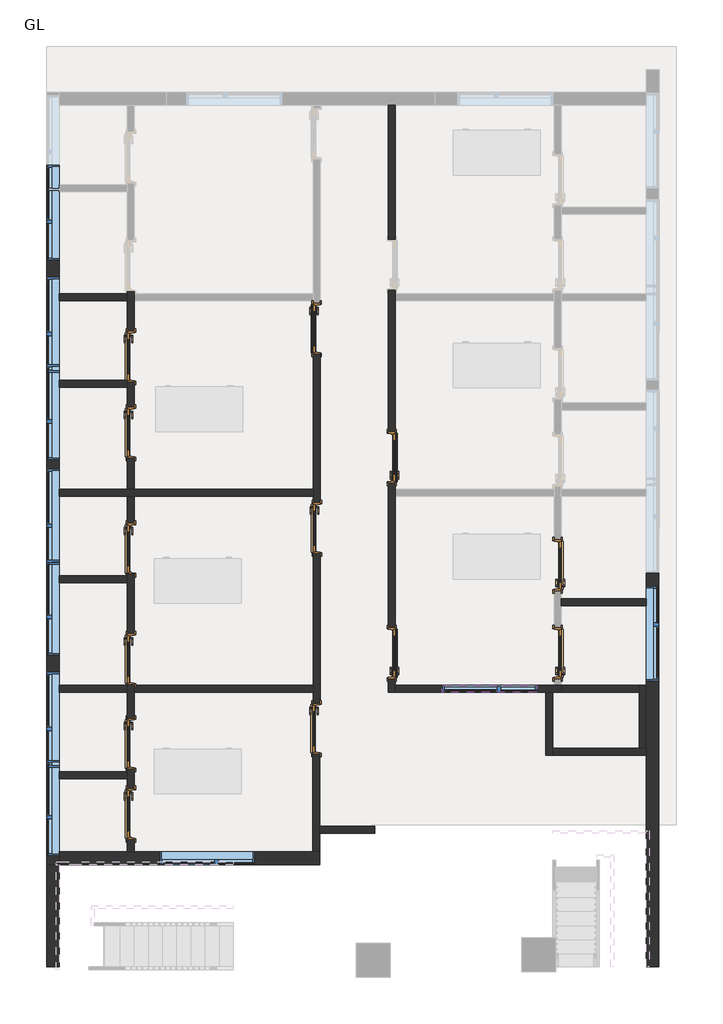
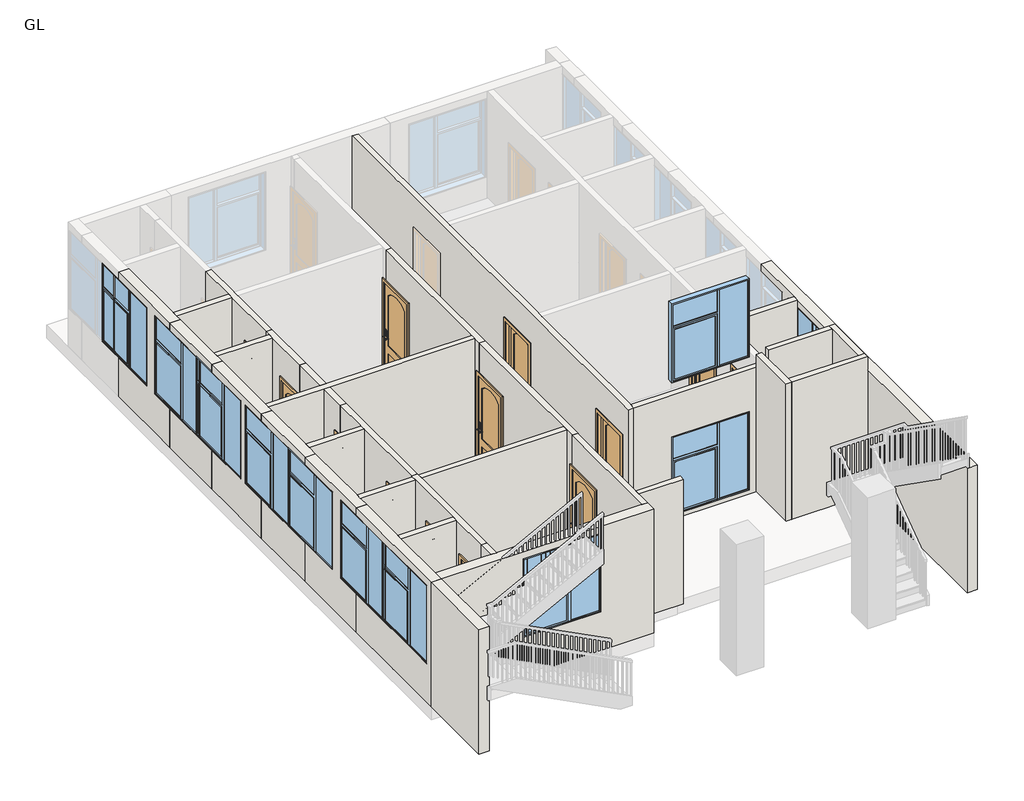
# One storey, part 1 of 4: 33 walls, 13 doors, 11 windows.
"""IFC4 building model written with IfcOpenShell, lengths in millimetres."""

from ifc_helpers import new_model, si_unit, frame, origin, origin_with_axes, place, context, project, spatial, polyline, outline, extrude, faceted_brep, transform, mapped, element, save
from components import door_346b4a94, m_window_casement_double_sidelight_1702_x_1829mm_c8b42c7f, m_window_casement_double_sidelight_1702_x_1829mm_92594323

model = new_model("IFC4")

# Units and contexts
model_context = context("Model", 3, world=origin())
ifc_project = project(units=[si_unit("LENGTHUNIT", "METRE", prefix="MILLI")], contexts=[model_context])

# Site, building, storey
site = spatial("IfcSite", under=ifc_project)
building = spatial("IfcBuilding", under=site)
storey = spatial("IfcBuildingStorey", under=building, Name="GL", Elevation=0.0)

# Doors
placement = place(None, origin())
door_shape = door_346b4a94(model_context)
element("IfcDoor", 1, ObjectType="2'10\"X7'", at=placement, inside=storey, context=model_context, shape_type="MappedRepresentation", body=[
    mapped(door_shape, transform((2698.7641134, -459.3600272, 0.0), x_axis=(0.0, -1.0, 0.0), y_axis=(1.0, 0.0, 0.0), z_axis=(0.0, 0.0, 1.0))),
])
element("IfcDoor", 2, ObjectType="2'10\"X7'", at=placement, inside=storey, context=model_context, shape_type="MappedRepresentation", body=[
    mapped(door_shape, transform((2698.7641134, -2034.1600272, 0.0), x_axis=(0.0, -1.0, 0.0), y_axis=(1.0, 0.0, 0.0), z_axis=(0.0, 0.0, 1.0))),
])
element("IfcDoor", 3, ObjectType="2'10\"X7'", at=placement, inside=storey, context=model_context, shape_type="MappedRepresentation", body=[
    mapped(door_shape, transform((-273.0358866, -2034.1600272, 0.0), x_axis=(0.0, -1.0, 0.0), y_axis=(1.0, 0.0, 0.0), z_axis=(0.0, 0.0, 1.0))),
])
element("IfcDoor", 4, ObjectType="2'10\"X7'", at=placement, inside=storey, context=model_context, shape_type="MappedRepresentation", body=[
    mapped(door_shape, transform((-273.0358866, 1471.0399728, 0.0), x_axis=(0.0, -1.0, 0.0), y_axis=(1.0, 0.0, 0.0), z_axis=(0.0, 0.0, 1.0))),
])
element("IfcDoor", 5, ObjectType="2'10\"X7'", at=placement, inside=storey, context=model_context, shape_type="MappedRepresentation", body=[
    mapped(door_shape, transform((-4952.9858866, -3659.7600272, 0.0), x_axis=(0.0, 1.0, 0.0), y_axis=(-1.0, 0.0, 0.0), z_axis=(0.0, 0.0, 1.0))),
])
element("IfcDoor", 6, ObjectType="2'10\"X7'", at=placement, inside=storey, context=model_context, shape_type="MappedRepresentation", body=[
    mapped(door_shape, transform((-4952.9858866, -2142.5151651, 0.0), x_axis=(0.0, 1.0, 0.0), y_axis=(-1.0, 0.0, 0.0), z_axis=(0.0, 0.0, 1.0))),
])
element("IfcDoor", 7, ObjectType="2'10\"X7'", at=placement, inside=storey, context=model_context, shape_type="MappedRepresentation", body=[
    mapped(door_shape, transform((-4952.9858866, -167.9704957, 0.0), x_axis=(0.0, 1.0, 0.0), y_axis=(-1.0, 0.0, 0.0), z_axis=(0.0, 0.0, 1.0))),
])
element("IfcDoor", 8, ObjectType="2'10\"X7'", at=placement, inside=storey, context=model_context, shape_type="MappedRepresentation", body=[
    mapped(door_shape, transform((-4952.9858866, 3273.6174518, 0.0), x_axis=(0.0, 1.0, 0.0), y_axis=(-1.0, 0.0, 0.0), z_axis=(0.0, 0.0, 1.0))),
])
element("IfcDoor", 9, ObjectType="2'10\"X7'", at=placement, inside=storey, context=model_context, shape_type="MappedRepresentation", body=[
    mapped(door_shape, transform((-1625.1621817, 3775.8008884, 0.0), x_axis=(0.0, 1.0, 0.0), y_axis=(-1.0, 0.0, 0.0), z_axis=(0.0, 0.0, 1.0))),
])
element("IfcDoor", 10, ObjectType="2'10\"X7'", at=placement, inside=storey, context=model_context, shape_type="MappedRepresentation", body=[
    mapped(door_shape, transform((-1629.1419858, -3390.4626067, 0.0), x_axis=(0.0, 1.0, 0.0), y_axis=(-1.0, 0.0, 0.0), z_axis=(0.0, 0.0, 1.0))),
])
element("IfcDoor", 11, ObjectType="2'10\"X7'", at=placement, inside=storey, context=model_context, shape_type="MappedRepresentation", body=[
    mapped(door_shape, transform((-1620.1577262, 202.9637706, 0.0), x_axis=(0.0, 1.0, 0.0), y_axis=(-1.0, 0.0, 0.0), z_axis=(0.0, 0.0, 1.0))),
])
element("IfcDoor", 12, ObjectType="2'10\"X7'", at=placement, inside=storey, context=model_context, shape_type="MappedRepresentation", body=[
    mapped(door_shape, transform((-4952.9858866, -4917.0600272, 0.0), x_axis=(0.0, 1.0, 0.0), y_axis=(-1.0, 0.0, 0.0), z_axis=(0.0, 0.0, 1.0))),
])
element("IfcDoor", 13, ObjectType="2'10\"X7'", at=placement, inside=storey, context=model_context, shape_type="MappedRepresentation", body=[
    mapped(door_shape, transform((-4952.9858866, 1913.3521609, 0.0), x_axis=(0.0, 1.0, 0.0), y_axis=(-1.0, 0.0, 0.0), z_axis=(0.0, 0.0, 1.0))),
])

# Walls
element("IfcWall", 14, ObjectType="Generic - 4.5\"", at=placement, inside=storey, context=model_context, shape_type="SweptSolid", body=[
    extrude(outline(polyline([(-5013.3108866, 4277.7399728), (-6232.5508078, 4277.7399728), (-6232.5508078, 4404.7399728), (-5013.3108866, 4404.7399728), (-5013.3108866, 4277.7399728)])), origin_with_axes(), (0.0, 0.0, 1.0), 2895.6),
])
element("IfcWall", 15, ObjectType="Generic - 4.5\"", at=placement, inside=storey, context=model_context, shape_type="Brep", body=[
    faceted_brep([(-5013.3108866, 2968.8174518, 2158.6), (-5013.3108866, 2968.8174518, 2895.6), (-5013.3108866, 4277.7399728, 2895.6), (-5013.3108866, 4404.7399728, 2895.6), (-5013.3108866, 5281.320652, 2895.6), (-5013.3108866, 5281.320652, 2158.6), (-5013.3108866, 4443.520652, 2158.6), (-5013.3108866, 4443.520652, 0.0), (-5013.3108866, 4404.7399728, 0.0), (-5013.3108866, 4277.7399728, 0.0), (-5013.3108866, 3730.4174518, 0.0), (-5013.3108866, 3730.4174518, 2158.6), (-4886.3108866, 2968.8174518, 2895.6), (-4886.3108866, 2968.8174518, 2158.6), (-4886.3108866, 3730.4174518, 2158.6), (-4886.3108866, 3730.4174518, 0.0), (-4886.3108866, 4277.7399728, 0.0), (-4886.3108866, 4404.7399728, 0.0), (-4886.3108866, 4443.520652, 0.0), (-4886.3108866, 4443.520652, 2158.6), (-4886.3108866, 5281.320652, 2158.6), (-4886.3108866, 5281.320652, 2895.6), (-4886.3108866, 4404.7399728, 2895.6), (-4886.3108866, 4277.7399728, 2895.6)], [[[0, 1, 2, 3, 4, 5, 6, 7, 8, 9, 10, 11]], [[12, 13, 14, 15, 16, 17, 18, 19, 20, 21, 22, 23]], [[15, 10, 9, 8, 7, 18, 17, 16]], [[1, 0, 13, 12]], [[4, 21, 20, 5]], [[14, 11, 10, 15]], [[11, 14, 13, 0]], [[19, 6, 5, 20]], [[6, 19, 18, 7]], [[4, 3, 2, 1, 12, 23, 22, 21]]]),
])
element("IfcWall", 16, ObjectType="Generic - 4.5\"", at=placement, inside=storey, context=model_context, shape_type="Brep", body=[
    faceted_brep([(-6232.5508078, 2728.3399728, 0.0), (-5013.3108866, 2728.3399728, 0.0), (-5013.3108866, 2728.3399728, 2895.6), (-6232.5508078, 2728.3399728, 2895.6), (-6232.5508078, 2855.3399728, 0.0), (-6232.5508078, 2855.3399728, 2895.6), (-5013.3108866, 2855.3399728, 2895.6), (-5013.3108866, 2855.3399728, 0.0), (-5013.3108866, 2816.8174518, 0.0)], [[[0, 1, 2, 3]], [[4, 5, 6, 7]], [[1, 0, 4, 7, 8]], [[0, 3, 5, 4]], [[2, 1, 8, 7, 6]], [[3, 2, 6, 5]]]),
])
element("IfcWall", 17, ObjectType="Generic - 4.5\"", at=placement, inside=storey, context=model_context, shape_type="Brep", body=[
    faceted_brep([(-5013.3108866, 2968.8174518, 2895.6), (-5013.3108866, 2968.8174518, 2158.6), (-5013.3108866, 2816.8174518, 2158.6), (-5013.3108866, 2816.8174518, 0.0), (-5013.3108866, 2728.3399728, 0.0), (-5013.3108866, 2370.1521609, 0.0), (-5013.3108866, 2370.1521609, 2158.6), (-5013.3108866, 1684.7521609, 2158.6), (-5013.3108866, 1684.7521609, 2895.6), (-5013.3108866, 2728.3399728, 2895.6), (-5013.3108866, 2855.3399728, 2895.6), (-4886.3108866, 2968.8174518, 2158.6), (-4886.3108866, 2968.8174518, 2895.6), (-4886.3108866, 1684.7521609, 2895.6), (-4886.3108866, 1684.7521609, 2158.6), (-4886.3108866, 2370.1521609, 2158.6), (-4886.3108866, 2370.1521609, 0.0), (-4886.3108866, 2816.8174518, 0.0), (-4886.3108866, 2816.8174518, 2158.6)], [[[0, 1, 2, 3, 4, 5, 6, 7, 8, 9, 10]], [[11, 12, 13, 14, 15, 16, 17, 18]], [[3, 17, 16, 5, 4]], [[13, 8, 7, 14]], [[1, 0, 12, 11]], [[18, 2, 1, 11]], [[2, 18, 17, 3]], [[15, 6, 5, 16]], [[6, 15, 14, 7]], [[0, 10, 9, 8, 13, 12]]]),
])
element("IfcWall", 18, ObjectType="Generic - 4.5\"", at=placement, inside=storey, context=model_context, shape_type="Brep", body=[
    faceted_brep([(-6232.5508078, 772.5399728, 0.0), (-5013.3108866, 772.5399728, 0.0), (-4886.3108866, 772.5399728, 0.0), (-1685.9108866, 772.5399728, 0.0), (-1685.9108866, 772.5399728, 2895.6), (-4886.3108866, 772.5399728, 2895.6), (-5013.3108866, 772.5399728, 2895.6), (-6232.5508078, 772.5399728, 2895.6), (-6232.5508078, 899.5399728, 0.0), (-6232.5508078, 899.5399728, 2895.6), (-5013.3108866, 899.5399728, 2895.6), (-4886.3108866, 899.5399728, 2895.6), (-1685.9108866, 899.5399728, 2895.6), (-1685.9108866, 899.5399728, 0.0), (-4886.3108866, 899.5399728, 0.0), (-5013.3108866, 899.5399728, 0.0)], [[[0, 1, 2, 3, 4, 5, 6, 7]], [[8, 9, 10, 11, 12, 13, 14, 15]], [[3, 2, 1, 0, 8, 15, 14, 13]], [[4, 3, 13, 12]], [[0, 7, 9, 8]], [[7, 6, 5, 4, 12, 11, 10, 9]]]),
])
element("IfcWall", 19, ObjectType="Generic - 4.5\"", at=placement, inside=storey, context=model_context, shape_type="SweptSolid", body=[
    extrude(outline(polyline([(136.8295043, 2158.6), (136.8295043, 2895.6), (772.5399728, 2895.6), (772.5399728, 0.0), (288.8295043, 0.0), (288.8295043, 2158.6), (136.8295043, 2158.6)])), frame((-5013.3108866, 0.0, 0.0), z_axis=(1.0, 0.0, 0.0), x_axis=(0.0, 1.0, 0.0)), (0.0, 0.0, 1.0), 127.0),
    extrude(outline(polyline([(1684.7521609, 2895.6), (1684.7521609, 2158.6), (1456.5521609, 2158.6), (1456.5521609, 0.0), (899.5399728, 0.0), (899.5399728, 2895.6), (1684.7521609, 2895.6)])), frame((-5013.3108866, 0.0, 0.0), z_axis=(1.0, 0.0, 0.0), x_axis=(0.0, 1.0, 0.0)), (0.0, 0.0, 1.0), 127.0),
])
element("IfcWall", 20, ObjectType="Generic - 4.5\"", at=placement, inside=storey, context=model_context, shape_type="SweptSolid", body=[
    extrude(outline(polyline([(-5013.3108866, -776.8600272), (-6232.5508078, -776.8600272), (-6232.5508078, -649.8600272), (-5013.3108866, -649.8600272), (-5013.3108866, -776.8600272)])), origin_with_axes(), (0.0, 0.0, 1.0), 2895.6),
])
element("IfcWall", 21, ObjectType="Generic - 4.5\"", at=placement, inside=storey, context=model_context, shape_type="Brep", body=[
    faceted_brep([(-5013.3108866, -2574.3151651, 2158.6), (-5013.3108866, -2574.3151651, 2895.6), (-5013.3108866, -776.8600272, 2895.6), (-5013.3108866, -649.8600272, 2895.6), (-5013.3108866, 136.8295043, 2895.6), (-5013.3108866, 136.8295043, 2158.6), (-5013.3108866, -624.7704957, 2158.6), (-5013.3108866, -624.7704957, 0.0), (-5013.3108866, -649.8600272, 0.0), (-5013.3108866, -776.8600272, 0.0), (-5013.3108866, -1685.7151651, 0.0), (-5013.3108866, -1685.7151651, 2158.6), (-4886.3108866, -2574.3151651, 2895.6), (-4886.3108866, -2574.3151651, 2158.6), (-4886.3108866, -1685.7151651, 2158.6), (-4886.3108866, -1685.7151651, 0.0), (-4886.3108866, -624.7704957, 0.0), (-4886.3108866, -624.7704957, 2158.6), (-4886.3108866, 136.8295043, 2158.6), (-4886.3108866, 136.8295043, 2895.6)], [[[0, 1, 2, 3, 4, 5, 6, 7, 8, 9, 10, 11]], [[12, 13, 14, 15, 16, 17, 18, 19]], [[15, 10, 9, 8, 7, 16]], [[1, 0, 13, 12]], [[4, 19, 18, 5]], [[14, 11, 10, 15]], [[11, 14, 13, 0]], [[17, 6, 5, 18]], [[6, 17, 16, 7]], [[4, 3, 2, 1, 12, 19]]]),
])
element("IfcWall", 22, ObjectType="Generic - 4.5\"", at=placement, inside=storey, context=model_context, shape_type="SweptSolid", body=[
    extrude(outline(polyline([(-5013.3108866, -2732.6600272), (-6232.5508078, -2732.6600272), (-6232.5508078, -2605.6600272), (-5013.3108866, -2605.6600272), (-5013.3108866, -2732.6600272)])), origin_with_axes(), (0.0, 0.0, 1.0), 2895.6),
])
element("IfcWall", 23, ObjectType="Generic - 4.5\"", at=placement, inside=storey, context=model_context, shape_type="Brep", body=[
    faceted_brep([(-5013.3108866, -3202.9600272, 0.0), (-5013.3108866, -3202.9600272, 2158.6), (-5013.3108866, -4116.5600272, 2158.6), (-5013.3108866, -4116.5600272, 0.0), (-5013.3108866, -4155.0600272, 0.0), (-5013.3108866, -4282.0600272, 0.0), (-5013.3108866, -4460.2600272, 0.0), (-5013.3108866, -4460.2600272, 2158.6), (-5013.3108866, -5221.8600272, 2158.6), (-5013.3108866, -5221.8600272, 2895.6), (-5013.3108866, -4282.0600272, 2895.6), (-5013.3108866, -4155.0600272, 2895.6), (-5013.3108866, -2732.6600272, 2895.6), (-5013.3108866, -2605.6600272, 2895.6), (-5013.3108866, -2574.3151651, 2895.6), (-5013.3108866, -2574.3151651, 2158.6), (-5013.3108866, -2599.3151651, 2158.6), (-5013.3108866, -2599.3151651, 0.0), (-5013.3108866, -2605.6600272, 0.0), (-5013.3108866, -2732.6600272, 0.0), (-4886.3108866, -3202.9600272, 2158.6), (-4886.3108866, -3202.9600272, 0.0), (-4886.3108866, -2732.6600272, 0.0), (-4886.3108866, -2605.6600272, 0.0), (-4886.3108866, -2599.3151651, 0.0), (-4886.3108866, -2599.3151651, 2158.6), (-4886.3108866, -2574.3151651, 2158.6), (-4886.3108866, -2574.3151651, 2895.6), (-4886.3108866, -2605.6600272, 2895.6), (-4886.3108866, -2732.6600272, 2895.6), (-4886.3108866, -5221.8600272, 2895.6), (-4886.3108866, -5221.8600272, 2158.6), (-4886.3108866, -4460.2600272, 2158.6), (-4886.3108866, -4460.2600272, 0.0), (-4886.3108866, -4116.5600272, 0.0), (-4886.3108866, -4116.5600272, 2158.6)], [[[0, 1, 2, 3, 4, 5, 6, 7, 8, 9, 10, 11, 12, 13, 14, 15, 16, 17, 18, 19]], [[20, 21, 22, 23, 24, 25, 26, 27, 28, 29, 30, 31, 32, 33, 34, 35]], [[21, 0, 19, 18, 17, 24, 23, 22]], [[3, 34, 33, 6, 5, 4]], [[30, 9, 8, 31]], [[15, 14, 27, 26]], [[20, 1, 0, 21]], [[1, 20, 35, 2]], [[2, 35, 34, 3]], [[25, 16, 15, 26]], [[16, 25, 24, 17]], [[32, 7, 6, 33]], [[7, 32, 31, 8]], [[14, 13, 12, 11, 10, 9, 30, 29, 28, 27]]]),
])
element("IfcWall", 24, ObjectType="Generic - 4.5\"", at=placement, inside=storey, context=model_context, shape_type="SweptSolid", body=[
    extrude(outline(polyline([(-5013.3108866, -4282.0600272), (-6232.5324766, -4282.0600272), (-6232.5342541, -4155.0600272), (-5013.3108866, -4155.0600272), (-5013.3108866, -4282.0600272)])), origin_with_axes(), (0.0, 0.0, 1.0), 2895.6),
])
element("IfcWall", 25, ObjectType="Generic - 4.5\"", at=placement, inside=storey, context=model_context, shape_type="SweptSolid", body=[
    extrude(outline(polyline([(-1685.9108866, -2732.6600272), (-4886.3108866, -2732.6600272), (-4886.3108866, -2605.6600272), (-1685.9108866, -2605.6600272), (-1685.9108866, -2732.6600272)])), origin_with_axes(), (0.0, 0.0, 1.0), 2895.6),
])
element("IfcWall", 26, ObjectType="Generic - 4.5\"", at=placement, inside=storey, context=model_context, shape_type="Brep", body=[
    faceted_brep([(-1685.4871817, 4182.2008884, 2895.6), (-1685.4871817, 4182.2008884, 2158.6), (-1685.4871817, 3319.0008884, 2158.6), (-1685.4871817, 3319.0008884, 0.0), (-1685.4871817, 659.7637706, 0.0), (-1685.4871817, 659.7637706, 2158.6), (-1685.4871817, 609.3637706, 2158.6), (-1685.4871817, 609.3637706, 2895.6), (-1558.4871817, 4182.2008884, 2158.6), (-1558.4871817, 4182.2008884, 2895.6), (-1558.4871817, 609.3637706, 2895.6), (-1558.4871817, 609.3637706, 2158.6), (-1558.4871817, 659.7637706, 2158.6), (-1558.4871817, 659.7637706, 0.0), (-1558.4871817, 3319.0008884, 0.0), (-1558.4871817, 3319.0008884, 2158.6), (-1680.4827262, 609.3637706, 2895.6), (-1680.4827262, 609.3637706, 2158.6), (-1558.9108866, 4182.2008884, 2895.6), (-1558.9108866, 4182.2008884, 2158.6)], [[[0, 1, 2, 3, 4, 5, 6, 7]], [[8, 9, 10, 11, 12, 13, 14, 15]], [[3, 14, 13, 4]], [[10, 16, 7, 6, 17, 11]], [[1, 0, 18, 9, 8, 19]], [[15, 2, 1, 19, 8]], [[2, 15, 14, 3]], [[12, 5, 4, 13]], [[5, 12, 11, 17, 6]], [[0, 7, 16, 10, 9, 18]]]),
])
element("IfcWall", 27, ObjectType="Generic - 4.5\"", at=placement, inside=storey, context=model_context, shape_type="Brep", body=[
    faceted_brep([(-1680.4827262, -2933.2626067, 0.0), (-1680.4827262, -2933.2626067, 2895.6), (-1680.4827262, 609.3637706, 2895.6), (-1680.4827262, 609.3637706, 2158.6), (-1680.4827262, -253.8362294, 2158.6), (-1680.4827262, -253.8362294, 0.0), (-1553.4827262, -2933.2626067, 2895.6), (-1553.4827262, -2933.2626067, 0.0), (-1553.4827262, -253.8362294, 0.0), (-1553.4827262, -253.8362294, 2158.6), (-1553.4827262, 609.3637706, 2158.6), (-1553.4827262, 609.3637706, 2895.6), (-1562.4669858, -2933.2626067, 0.0), (-1562.4669858, -2933.2626067, 2895.6), (-1558.4871817, 609.3637706, 2895.6), (-1558.4871817, 609.3637706, 2158.6)], [[[0, 1, 2, 3, 4, 5]], [[6, 7, 8, 9, 10, 11]], [[7, 12, 0, 5, 8]], [[1, 0, 12, 7, 6, 13]], [[2, 14, 11, 10, 15, 3]], [[9, 4, 3, 15, 10]], [[4, 9, 8, 5]], [[2, 1, 13, 6, 11, 14]]]),
])
element("IfcWall", 28, ObjectType="Generic - 4.5\"", at=placement, inside=storey, context=model_context, shape_type="Brep", body=[
    faceted_brep([(-1689.4669858, -2933.2626067, 2895.6), (-1689.4669858, -2933.2626067, 0.0), (-1689.4669858, -2933.6626067, 0.0), (-1689.4669858, -2933.6626067, 2158.6), (-1689.4669858, -3847.2626067, 2158.6), (-1689.4669858, -3847.2626067, 0.0), (-1689.4669858, -5596.1082131, 0.0), (-1689.4669858, -5596.1082131, 2895.6), (-1562.4669858, -2933.2626067, 0.0), (-1562.4669858, -2933.2626067, 2895.6), (-1562.4669858, -5136.3822004, 2895.6), (-1562.4669858, -5263.3822004, 2895.6), (-1562.4669858, -5596.1082131, 2895.6), (-1562.4669858, -5596.1082131, 0.0), (-1562.4669858, -5263.3822004, 0.0), (-1562.4669858, -5136.3822004, 0.0), (-1562.4669858, -3847.2626067, 0.0), (-1562.4669858, -3847.2626067, 2158.6), (-1562.4669858, -2933.6626067, 2158.6), (-1562.4669858, -2933.6626067, 0.0), (-1680.4827262, -2933.2626067, 0.0), (-1680.4827262, -2933.2626067, 2895.6)], [[[0, 1, 2, 3, 4, 5, 6, 7]], [[8, 9, 10, 11, 12, 13, 14, 15, 16, 17, 18, 19]], [[1, 20, 8, 19, 2]], [[13, 6, 5, 16, 15, 14]], [[1, 0, 21, 9, 8, 20]], [[18, 3, 2, 19]], [[3, 18, 17, 4]], [[4, 17, 16, 5]], [[7, 6, 13, 12]], [[0, 7, 12, 11, 10, 9, 21]]]),
])
element("IfcWall", 29, ObjectType="Generic - 4.5\"", at=placement, inside=storey, context=model_context, shape_type="Brep", body=[
    faceted_brep([(-339.7108866, 7782.9399728, 2895.6), (-339.7108866, 7782.9399728, 0.0), (-339.7108866, 5382.2399728, 0.0), (-339.7108866, 5382.2399728, 2158.6), (-339.7108866, 4468.6399728, 2158.6), (-339.7108866, 4468.6399728, 0.0), (-339.7108866, 1927.8399728, 0.0), (-339.7108866, 1927.8399728, 2158.6), (-339.7108866, 1014.2399728, 2158.6), (-339.7108866, 1014.2399728, 0.0), (-339.7108866, -1577.3600272, 0.0), (-339.7108866, -1577.3600272, 2158.6), (-339.7108866, -2490.9600272, 2158.6), (-339.7108866, -2490.9600272, 0.0), (-339.7108866, -2732.6600272, 0.0), (-339.7108866, -2732.6600272, 2895.6), (-212.7108866, 7782.9399728, 0.0), (-212.7108866, 7782.9399728, 2895.6), (-212.7108866, 4404.7399728, 2895.6), (-212.7108866, 4277.7399728, 2895.6), (-212.7108866, 899.5399728, 2895.6), (-212.7108866, 772.5399728, 2895.6), (-212.7108866, -2605.6600272, 2895.6), (-212.7108866, -2732.6600272, 2895.6), (-212.7108866, -2732.6600272, 0.0), (-212.7108866, -2605.6600272, 0.0), (-212.7108866, -2490.9600272, 0.0), (-212.7108866, -2490.9600272, 2158.6), (-212.7108866, -1577.3600272, 2158.6), (-212.7108866, -1577.3600272, 0.0), (-212.7108866, 772.5399728, 0.0), (-212.7108866, 899.5399728, 0.0), (-212.7108866, 1014.2399728, 0.0), (-212.7108866, 1014.2399728, 2158.6), (-212.7108866, 1927.8399728, 2158.6), (-212.7108866, 1927.8399728, 0.0), (-212.7108866, 4277.7399728, 0.0), (-212.7108866, 4404.7399728, 0.0), (-212.7108866, 4468.6399728, 0.0), (-212.7108866, 4468.6399728, 2158.6), (-212.7108866, 5382.2399728, 2158.6), (-212.7108866, 5382.2399728, 0.0)], [[[0, 1, 2, 3, 4, 5, 6, 7, 8, 9, 10, 11, 12, 13, 14, 15]], [[16, 17, 18, 19, 20, 21, 22, 23, 24, 25, 26, 27, 28, 29, 30, 31, 32, 33, 34, 35, 36, 37, 38, 39, 40, 41]], [[1, 16, 41, 2]], [[24, 14, 13, 26, 25]], [[29, 10, 9, 32, 31, 30]], [[35, 6, 5, 38, 37, 36]], [[1, 0, 17, 16]], [[15, 14, 24, 23]], [[12, 27, 26, 13]], [[27, 12, 11, 28]], [[28, 11, 10, 29]], [[8, 33, 32, 9]], [[33, 8, 7, 34]], [[34, 7, 6, 35]], [[4, 39, 38, 5]], [[39, 4, 3, 40]], [[40, 3, 2, 41]], [[0, 15, 23, 22, 21, 20, 19, 18, 17]]]),
])
element("IfcWall", 30, ObjectType="Generic - 4.5\"", at=placement, inside=storey, context=model_context, shape_type="Brep", body=[
    faceted_brep([(-212.7108866, -2732.6600272, 0.0), (2479.6891134, -2732.6600272, 0.0), (2606.6891134, -2732.6600272, 0.0), (2759.0891134, -2732.6600272, 0.0), (2759.0891134, -2732.6600272, 2895.6), (-212.7108866, -2732.6600272, 2895.6), (625.4891134, -2732.6600272, 1925.9883506), (2327.2891134, -2732.6600272, 1925.9883506), (2327.2891134, -2732.6600272, 97.1883506), (625.4891134, -2732.6600272, 97.1883506), (-212.7108866, -2605.6600272, 0.0), (-212.7108866, -2605.6600272, 2895.6), (2632.0891134, -2605.6600272, 2895.6), (2759.0891134, -2605.6600272, 2895.6), (2759.0891134, -2605.6600272, 0.0), (2632.0891134, -2605.6600272, 0.0), (625.4891134, -2605.6600272, 1925.9883506), (625.4891134, -2605.6600272, 97.1883506), (2327.2891134, -2605.6600272, 97.1883506), (2327.2891134, -2605.6600272, 1925.9883506)], [[[0, 1, 2, 3, 4, 5], [6, 7, 8, 9]], [[10, 11, 12, 13, 14, 15], [16, 17, 18, 19]], [[3, 2, 1, 0, 10, 15, 14]], [[0, 5, 11, 10]], [[5, 4, 13, 12, 11]], [[17, 16, 6, 9]], [[18, 17, 9, 8]], [[19, 18, 8, 7]], [[16, 19, 7, 6]], [[4, 3, 14, 13]]]),
])
element("IfcWall", 31, ObjectType="Generic - 4.5\"", at=placement, inside=storey, context=model_context, shape_type="SweptSolid", body=[
    extrude(outline(polyline([(4281.7311655, -1183.2600272), (2759.0891134, -1183.2600272), (2759.0891134, -1056.2600272), (4281.7311655, -1056.2600272), (4281.7311655, -1183.2600272)])), origin_with_axes(), (0.0, 0.0, 1.0), 2895.6),
])
element("IfcWall", 32, ObjectType="Generic - 5\"", at=placement, inside=storey, context=model_context, shape_type="SweptSolid", body=[
    extrude(outline(polyline([(-5593.5822004, 0.0), (-5593.5822004, 2895.6), (-5221.8600272, 2895.6), (-5221.8600272, 2158.6), (-5373.8600272, 2158.6), (-5373.8600272, 0.0), (-5593.5822004, 0.0)])), frame((-5013.3108866, 0.0, 0.0), z_axis=(1.0, 0.0, 0.0), x_axis=(0.0, 1.0, 0.0)), (0.0, 0.0, 1.0), 127.0),
])
element("IfcWall", 33, ObjectType="Generic - 5\"", at=placement, inside=storey, context=model_context, shape_type="SweptSolid", body=[
    extrude(outline(polyline([(-1562.4669858, -5136.3822004), (-581.0108866, -5136.3822004), (-581.0108866, -5263.3822004), (-1562.4669858, -5263.3822004), (-1562.4669858, -5136.3822004)])), origin_with_axes(), (0.0, 0.0, 1.0), 2895.6),
])
element("IfcWall", 34, ObjectType="Generic - 5\"", at=placement, inside=storey, context=model_context, shape_type="Brep", body=[
    faceted_brep([(2479.6891134, -2732.6600272, 0.0), (2479.6891134, -3866.3822004, 0.0), (2479.6891134, -3866.3822004, 3200.4), (2479.6891134, -2732.6600272, 3200.4), (2606.6891134, -2732.6600272, 0.0), (2606.6891134, -2732.6600272, 3200.4), (2606.6891134, -3739.3822004, 3200.4), (2606.6891134, -3866.3822004, 3200.4), (2606.6891134, -3866.3822004, 0.0), (2606.6891134, -3739.3822004, 0.0)], [[[0, 1, 2, 3]], [[4, 5, 6, 7, 8, 9]], [[1, 0, 4, 9, 8]], [[3, 2, 7, 6, 5]], [[0, 3, 5, 4]], [[2, 1, 8, 7]]]),
])
element("IfcWall", 35, ObjectType="Generic - 5\"", at=placement, inside=storey, context=model_context, shape_type="Brep", body=[
    faceted_brep([(2606.6891134, -3866.3822004, 0.0), (4281.7311655, -3866.3822004, 0.0), (4281.7311655, -3866.3822004, 3200.4), (2606.6891134, -3866.3822004, 3200.4), (2606.6891134, -3739.3822004, 0.0), (2606.6891134, -3739.3822004, 3200.4), (4154.7311655, -3739.3822004, 3200.4), (4281.7311655, -3739.3822004, 3200.4), (4281.7311655, -3739.3822004, 0.0), (4154.7311655, -3739.3822004, 0.0)], [[[0, 1, 2, 3]], [[4, 5, 6, 7, 8, 9]], [[1, 0, 4, 9, 8]], [[3, 2, 7, 6, 5]], [[0, 3, 5, 4]], [[2, 1, 8, 7]]]),
])
element("IfcWall", 36, ObjectType="Generic - 5\"", at=placement, inside=storey, context=model_context, shape_type="Brep", body=[
    faceted_brep([(4281.7311655, -3739.3822004, 0.0), (4281.7311655, -2605.6600272, 0.0), (4281.7311655, -2605.6600272, 3200.4), (4281.7311655, -3739.3822004, 3200.4), (4154.7311655, -3739.3822004, 0.0), (4154.7311655, -3739.3822004, 3200.4), (4154.7311655, -2732.6600272, 3200.4), (4154.7311655, -2605.6600272, 3200.4), (4154.7311655, -2605.6600272, 0.0), (4154.7311655, -2732.6600272, 0.0)], [[[0, 1, 2, 3]], [[4, 5, 6, 7, 8, 9]], [[1, 0, 4, 9, 8]], [[3, 2, 7, 6, 5]], [[0, 3, 5, 4]], [[2, 1, 8, 7]]]),
])
element("IfcWall", 37, ObjectType="Generic - 5\"", at=placement, inside=storey, context=model_context, shape_type="Brep", body=[
    faceted_brep([(2759.0891134, -2732.6600272, 0.0), (4154.7311655, -2732.6600272, 0.0), (4154.7311655, -2732.6600272, 3200.4), (2759.0891134, -2732.6600272, 3200.4), (2759.0891134, -2732.6600272, 2895.6), (2759.0891134, -2605.6600272, 0.0), (2759.0891134, -2605.6600272, 2895.6), (2759.0891134, -2605.6600272, 3200.4), (4154.7311655, -2605.6600272, 3200.4), (4154.7311655, -2605.6600272, 0.0)], [[[0, 1, 2, 3, 4]], [[5, 6, 7, 8, 9]], [[1, 0, 5, 9]], [[3, 2, 8, 7]], [[2, 1, 9, 8]], [[0, 4, 3, 7, 6, 5]]]),
])
element("IfcWall", 38, ObjectType="Generic - 9\"", at=placement, inside=storey, context=model_context, shape_type="Brep", body=[
    faceted_brep([(4281.7311655, 200.5184135, 0.0), (4281.7311655, -1056.2600272, 0.0), (4281.7311655, -1183.2600272, 0.0), (4281.7311655, -7650.9822004, 0.0), (4281.7311655, -7650.9822004, 2895.6), (4281.7311655, -1183.2600272, 2895.6), (4281.7311655, -1056.2600272, 2895.6), (4281.7311655, 200.5184135, 2895.6), (4281.7311655, 200.5184135, 2728.8), (4281.7311655, -599.0600272, 2728.8), (4281.7311655, -599.0600272, 900.0), (4281.7311655, 200.5184135, 900.0), (4281.7311655, -2537.537179, 900.0), (4281.7311655, -835.737179, 900.0), (4281.7311655, -835.737179, 2728.8), (4281.7311655, -2537.537179, 2728.8), (4510.3311655, -7650.9822004, 0.0), (4510.3311655, 200.5184135, 0.0), (4510.3311655, 200.5184135, 900.0), (4510.3311655, -599.0600272, 900.0), (4510.3311655, -599.0600272, 2728.8), (4510.3311655, 200.5184135, 2728.8), (4510.3311655, 200.5184135, 2895.6), (4510.3311655, -7650.9822004, 2895.6), (4510.3311655, -835.737179, 900.0), (4510.3311655, -2537.537179, 900.0), (4510.3311655, -2537.537179, 2728.8), (4510.3311655, -835.737179, 2728.8), (4283.0918814, 200.5184135, 0.0), (4283.0918814, 200.5184135, 900.0), (4283.0918814, 200.5184135, 2895.6), (4283.0918814, 200.5184135, 2728.8)], [[[0, 1, 2, 3, 4, 5, 6, 7, 8, 9, 10, 11], [12, 13, 14, 15]], [[16, 17, 18, 19, 20, 21, 22, 23], [24, 25, 26, 27]], [[3, 2, 1, 0, 28, 17, 16]], [[4, 3, 16, 23]], [[17, 28, 0, 11, 29, 18]], [[8, 7, 30, 22, 21, 31]], [[9, 20, 19, 10]], [[10, 19, 18, 29, 11]], [[20, 9, 8, 31, 21]], [[24, 13, 12, 25]], [[13, 24, 27, 14]], [[14, 27, 26, 15]], [[25, 12, 15, 26]], [[7, 6, 5, 4, 23, 22, 30]]]),
])
element("IfcWall", 39, ObjectType="Generic - 9\"", at=placement, inside=storey, context=model_context, shape_type="Brep", body=[
    faceted_brep([(-6232.5108866, -5824.7082131, 0.0), (-6232.5140859, -5596.1082131, 0.0), (-6232.5324766, -4282.0600272, 0.0), (-6232.5342541, -4155.0600272, 0.0), (-6232.5508078, -2972.263382, 0.0), (-6232.5508078, -2972.263382, 900.0), (-6232.5131972, -5659.6082132, 900.0), (-6232.5131972, -5659.6082132, 2728.8), (-6232.5508078, -2972.263382, 2728.8), (-6232.5508078, -2972.263382, 2895.6), (-6232.5342541, -4155.0600272, 2895.6), (-6232.5324766, -4282.0600272, 2895.6), (-6232.5140859, -5596.1082131, 2895.6), (-6232.5108866, -5824.7082131, 2895.6), (-6461.1508078, -2972.2665814, 0.0), (-6461.1108866, -5824.7082131, 0.0), (-6461.1108866, -5824.7082131, 2895.6), (-6461.1508078, -2972.2665814, 2895.6), (-6461.1508078, -2972.2665814, 2728.8), (-6461.1131972, -5659.6114126, 2728.8), (-6461.1131972, -5659.6114126, 900.0), (-6461.1508078, -2972.2665814, 900.0)], [[[0, 1, 2, 3, 4, 5, 6, 7, 8, 9, 10, 11, 12, 13]], [[14, 15, 16, 17, 18, 19, 20, 21]], [[4, 3, 2, 1, 0, 15, 14]], [[4, 14, 21, 5]], [[9, 8, 18, 17]], [[5, 21, 20, 6]], [[18, 8, 7, 19]], [[19, 7, 6, 20]], [[0, 13, 16, 15]], [[13, 12, 11, 10, 9, 17, 16]]]),
])
element("IfcWall", 40, ObjectType="Generic - 9\"", at=placement, inside=storey, context=model_context, shape_type="Brep", body=[
    faceted_brep([(-6232.5508078, -2972.2649817, 0.0), (-6232.5508078, -2732.6600272, 0.0), (-6232.5508078, -2605.6600272, 0.0), (-6232.5508078, -1019.7048138, 0.0), (-6232.5508078, -1019.7048138, 900.0), (-6232.5508078, -2073.8048138, 900.0), (-6232.5508078, -2073.8048138, 2728.8), (-6232.5508078, -1019.7048138, 2728.8), (-6232.5508078, -1019.7048138, 2895.6), (-6232.5508078, -2605.6600272, 2895.6), (-6232.5508078, -2732.6600272, 2895.6), (-6232.5508078, -2972.2649817, 2895.6), (-6232.5508078, -2972.2649817, 2728.8), (-6232.5508078, -2375.3633819, 2728.8), (-6232.5508078, -2375.3633819, 900.0), (-6232.5508078, -2972.2649817, 900.0), (-6461.1508078, -1019.7048138, 0.0), (-6461.1508078, -2972.2649817, 0.0), (-6461.1508078, -2972.2649817, 900.0), (-6461.1508078, -2375.3665813, 900.0), (-6461.1508078, -2375.3665813, 2728.8), (-6461.1508078, -2972.2649817, 2728.8), (-6461.1508078, -2972.2649817, 2895.6), (-6461.1508078, -1019.7048138, 2895.6), (-6461.1508078, -1019.7048138, 2728.8), (-6461.1508078, -2073.8048138, 2728.8), (-6461.1508078, -2073.8048138, 900.0), (-6461.1508078, -1019.7048138, 900.0)], [[[0, 1, 2, 3, 4, 5, 6, 7, 8, 9, 10, 11, 12, 13, 14, 15]], [[16, 17, 18, 19, 20, 21, 22, 23, 24, 25, 26, 27]], [[3, 2, 1, 0, 17, 16]], [[3, 16, 27, 4]], [[8, 7, 24, 23]], [[17, 0, 15, 18]], [[11, 22, 21, 12]], [[26, 5, 4, 27]], [[5, 26, 25, 6]], [[6, 25, 24, 7]], [[13, 20, 19, 14]], [[14, 19, 18, 15]], [[20, 13, 12, 21]], [[11, 10, 9, 8, 23, 22]]]),
])
element("IfcWall", 41, ObjectType="Generic - 9\"", at=placement, inside=storey, context=model_context, shape_type="Brep", body=[
    faceted_brep([(-6232.5508078, -1019.7048138, 0.0), (-6232.5508078, -776.8600272, 0.0), (-6232.5508078, -649.8600272, 0.0), (-6232.5508078, 642.0011338, 0.0), (-6232.5508078, 642.0011338, 900.0), (-6232.5508078, -1019.7048138, 900.0), (-6461.1508078, 642.0011338, 0.0), (-6461.1508078, -1019.7048138, 0.0), (-6461.1508078, -1019.7048138, 900.0), (-6461.1508078, 642.0011338, 900.0)], [[[0, 1, 2, 3, 4, 5]], [[6, 7, 8, 9]], [[3, 2, 1, 0, 7, 6]], [[3, 6, 9, 4]], [[7, 0, 5, 8]], [[4, 9, 8, 5]]]),
    faceted_brep([(-6232.5508078, -1019.7048138, 2728.8), (-6232.5508078, 642.0011338, 2728.8), (-6232.5508078, 642.0011338, 2895.6), (-6232.5508078, -649.8600272, 2895.6), (-6232.5508078, -776.8600272, 2895.6), (-6232.5508078, -1019.7048138, 2895.6), (-6461.1508078, 642.0011338, 2895.6), (-6461.1508078, 642.0011338, 2728.8), (-6461.1508078, -1019.7048138, 2728.8), (-6461.1508078, -1019.7048138, 2895.6)], [[[0, 1, 2, 3, 4, 5]], [[6, 7, 8, 9]], [[2, 1, 7, 6]], [[5, 9, 8, 0]], [[7, 1, 0, 8]], [[5, 4, 3, 2, 6, 9]]]),
])
element("IfcWall", 42, ObjectType="Generic - 9\"", at=placement, inside=storey, context=model_context, shape_type="Brep", body=[
    faceted_brep([(-6232.5508078, 642.0011338, 0.0), (-6232.5508078, 772.5399728, 0.0), (-6232.5508078, 899.5399728, 0.0), (-6232.5508078, 2534.5107865, 0.0), (-6232.5508078, 2534.5107865, 900.0), (-6232.5508078, 1429.6107865, 900.0), (-6232.5508078, 1429.6107865, 2728.8), (-6232.5508078, 2534.5107865, 2728.8), (-6232.5508078, 2534.5107865, 2895.6), (-6232.5508078, 899.5399728, 2895.6), (-6232.5508078, 772.5399728, 2895.6), (-6232.5508078, 642.0011338, 2895.6), (-6232.5508078, 642.0011338, 2728.8), (-6232.5508078, 1264.3011338, 2728.8), (-6232.5508078, 1264.3011338, 900.0), (-6232.5508078, 642.0011338, 900.0), (-6461.1508078, 2534.5107865, 0.0), (-6461.1508078, 642.0011338, 0.0), (-6461.1508078, 642.0011338, 900.0), (-6461.1508078, 1264.3011338, 900.0), (-6461.1508078, 1264.3011338, 2728.8), (-6461.1508078, 642.0011338, 2728.8), (-6461.1508078, 642.0011338, 2895.6), (-6461.1508078, 2534.5107865, 2895.6), (-6461.1508078, 2534.5107865, 2728.8), (-6461.1508078, 1429.6107865, 2728.8), (-6461.1508078, 1429.6107865, 900.0), (-6461.1508078, 2534.5107865, 900.0)], [[[0, 1, 2, 3, 4, 5, 6, 7, 8, 9, 10, 11, 12, 13, 14, 15]], [[16, 17, 18, 19, 20, 21, 22, 23, 24, 25, 26, 27]], [[3, 2, 1, 0, 17, 16]], [[3, 16, 27, 4]], [[8, 7, 24, 23]], [[17, 0, 15, 18]], [[11, 22, 21, 12]], [[26, 5, 4, 27]], [[5, 26, 25, 6]], [[6, 25, 24, 7]], [[13, 20, 19, 14]], [[14, 19, 18, 15]], [[20, 13, 12, 21]], [[11, 10, 9, 8, 23, 22]]]),
])
element("IfcWall", 43, ObjectType="Generic - 9\"", at=placement, inside=storey, context=model_context, shape_type="Brep", body=[
    faceted_brep([(-6232.5508078, 2534.5107865, 0.0), (-6232.5508078, 2728.3399728, 0.0), (-6232.5508078, 2855.3399728, 0.0), (-6232.5508078, 4130.2388609, 0.0), (-6232.5508078, 4130.2388609, 900.0), (-6232.5508078, 2534.5107865, 900.0), (-6461.1508078, 4130.2388609, 0.0), (-6461.1508078, 2534.5107865, 0.0), (-6461.1508078, 2534.5107865, 900.0), (-6461.1508078, 4130.2388609, 900.0)], [[[0, 1, 2, 3, 4, 5]], [[6, 7, 8, 9]], [[3, 2, 1, 0, 7, 6]], [[3, 6, 9, 4]], [[7, 0, 5, 8]], [[4, 9, 8, 5]]]),
    faceted_brep([(-6232.5508078, 2534.5107865, 2728.8), (-6232.5508078, 4130.2388609, 2728.8), (-6232.5508078, 4130.2388609, 2895.6), (-6232.5508078, 2855.3399728, 2895.6), (-6232.5508078, 2728.3399728, 2895.6), (-6232.5508078, 2534.5107865, 2895.6), (-6461.1508078, 4130.2388609, 2895.6), (-6461.1508078, 4130.2388609, 2728.8), (-6461.1508078, 2534.5107865, 2728.8), (-6461.1508078, 2534.5107865, 2895.6)], [[[0, 1, 2, 3, 4, 5]], [[6, 7, 8, 9]], [[2, 1, 7, 6]], [[5, 9, 8, 0]], [[7, 1, 0, 8]], [[5, 4, 3, 2, 6, 9]]]),
])
element("IfcWall", 44, ObjectType="Generic - 9\"", at=placement, inside=storey, context=model_context, shape_type="Brep", body=[
    faceted_brep([(-6232.5508078, 4130.2388609, 0.0), (-6232.5508078, 4277.7399728, 0.0), (-6232.5508078, 4404.7399728, 0.0), (-6232.5508078, 6088.0863192, 0.0), (-6232.5508078, 6088.0863192, 900.0), (-6232.5508078, 5008.5863192, 900.0), (-6232.5508078, 5008.5863192, 2728.8), (-6232.5508078, 6088.0863192, 2728.8), (-6232.5508078, 6088.0863192, 2895.6), (-6232.5508078, 4404.7399728, 2895.6), (-6232.5508078, 4277.7399728, 2895.6), (-6232.5508078, 4130.2388609, 2895.6), (-6232.5508078, 4130.2388609, 2728.8), (-6232.5508078, 4701.7388609, 2728.8), (-6232.5508078, 4701.7388609, 900.0), (-6232.5508078, 4130.2388609, 900.0), (-6461.1508078, 6088.0863192, 0.0), (-6461.1508078, 4130.2388609, 0.0), (-6461.1508078, 4130.2388609, 900.0), (-6461.1508078, 4701.7388609, 900.0), (-6461.1508078, 4701.7388609, 2728.8), (-6461.1508078, 4130.2388609, 2728.8), (-6461.1508078, 4130.2388609, 2895.6), (-6461.1508078, 6088.0863192, 2895.6), (-6461.1508078, 6088.0863192, 2728.8), (-6461.1508078, 5008.5863192, 2728.8), (-6461.1508078, 5008.5863192, 900.0), (-6461.1508078, 6088.0863192, 900.0)], [[[0, 1, 2, 3, 4, 5, 6, 7, 8, 9, 10, 11, 12, 13, 14, 15]], [[16, 17, 18, 19, 20, 21, 22, 23, 24, 25, 26, 27]], [[3, 2, 1, 0, 17, 16]], [[3, 16, 27, 4]], [[8, 7, 24, 23]], [[17, 0, 15, 18]], [[11, 22, 21, 12]], [[26, 5, 4, 27]], [[5, 26, 25, 6]], [[6, 25, 24, 7]], [[13, 20, 19, 14]], [[14, 19, 18, 15]], [[20, 13, 12, 21]], [[11, 10, 9, 8, 23, 22]]]),
])
element("IfcWall", 45, ObjectType="Generic - 9\"", at=placement, inside=storey, context=model_context, shape_type="Brep", body=[
    faceted_brep([(-6232.5108866, -5824.7082131, 0.0), (-1562.4669858, -5824.7082131, 0.0), (-1562.4669858, -5824.7082131, 2895.6), (-6232.5108866, -5824.7082131, 2895.6), (-4432.6669858, -5824.7082131, 2728.8), (-2730.8669858, -5824.7082131, 2728.8), (-2730.8669858, -5824.7082131, 900.0), (-4432.6669858, -5824.7082131, 900.0), (-6232.5140859, -5596.1082131, 0.0), (-6232.5140859, -5596.1082131, 2895.6), (-1689.4669858, -5596.1082131, 2895.6), (-1562.4669858, -5596.1082131, 2895.6), (-1562.4669858, -5596.1082131, 0.0), (-1689.4669858, -5596.1082131, 0.0), (-4432.6669858, -5596.1082131, 2728.8), (-4432.6669858, -5596.1082131, 900.0), (-2730.8669858, -5596.1082131, 900.0), (-2730.8669858, -5596.1082131, 2728.8)], [[[0, 1, 2, 3], [4, 5, 6, 7]], [[8, 9, 10, 11, 12, 13], [14, 15, 16, 17]], [[1, 0, 8, 13, 12]], [[2, 1, 12, 11]], [[0, 3, 9, 8]], [[3, 2, 11, 10, 9]], [[15, 14, 4, 7]], [[16, 15, 7, 6]], [[17, 16, 6, 5]], [[14, 17, 5, 4]]]),
])
element("IfcWall", 46, ObjectType="Generic - 9\"", at=placement, inside=storey, context=model_context, shape_type="SweptSolid", body=[
    extrude(outline(polyline([(-6461.1131972, -7650.9822004), (-6461.1131972, -5824.7082131), (-6232.5131972, -5824.7082131), (-6232.5131972, -7650.9822004), (-6461.1131972, -7650.9822004)])), origin_with_axes(), (0.0, 0.0, 1.0), 2895.6),
])

# Windows
m_window_casement_double_sidelight_1702_x_1829mm_shape = m_window_casement_double_sidelight_1702_x_1829mm_c8b42c7f(model_context)
element("IfcWindow", 47, ObjectType="M_Window-Casement-Double-Sidelight : 1702 x 1829mm", at=placement, inside=storey, context=model_context, shape_type="MappedRepresentation", body=[
    mapped(m_window_casement_double_sidelight_1702_x_1829mm_shape, transform((-6346.8508078, 5859.4863192, 0.0), x_axis=(0.0, 1.0, 0.0), y_axis=(-1.0, 0.0, 0.0), z_axis=(0.0, 0.0, 1.0))),
])
element("IfcWindow", 48, ObjectType="M_Window-Casement-Double-Sidelight : 1702 x 1829mm", at=placement, inside=storey, context=model_context, shape_type="MappedRepresentation", body=[
    mapped(m_window_casement_double_sidelight_1702_x_1829mm_shape, transform((-6346.8508078, 3850.8388609, 0.0), x_axis=(0.0, 1.0, 0.0), y_axis=(-1.0, 0.0, 0.0), z_axis=(0.0, 0.0, 1.0))),
])
element("IfcWindow", 49, ObjectType="M_Window-Casement-Double-Sidelight : 1702 x 1829mm", at=placement, inside=storey, context=model_context, shape_type="MappedRepresentation", body=[
    mapped(m_window_casement_double_sidelight_1702_x_1829mm_shape, transform((-6346.8508078, 2280.5107865, 0.0), x_axis=(0.0, 1.0, 0.0), y_axis=(-1.0, 0.0, 0.0), z_axis=(0.0, 0.0, 1.0))),
])
element("IfcWindow", 50, ObjectType="M_Window-Casement-Double-Sidelight : 1702 x 1829mm", at=placement, inside=storey, context=model_context, shape_type="MappedRepresentation", body=[
    mapped(m_window_casement_double_sidelight_1702_x_1829mm_shape, transform((-6346.8508078, 413.4011338, 0.0), x_axis=(0.0, 1.0, 0.0), y_axis=(-1.0, 0.0, 0.0), z_axis=(0.0, 0.0, 1.0))),
])
element("IfcWindow", 51, ObjectType="M_Window-Casement-Double-Sidelight : 1702 x 1829mm", at=placement, inside=storey, context=model_context, shape_type="MappedRepresentation", body=[
    mapped(m_window_casement_double_sidelight_1702_x_1829mm_shape, transform((-6346.8508078, -1222.9048138, 0.0), x_axis=(0.0, 1.0, 0.0), y_axis=(-1.0, 0.0, 0.0), z_axis=(0.0, 0.0, 1.0))),
])
element("IfcWindow", 52, ObjectType="M_Window-Casement-Double-Sidelight : 1702 x 1829mm", at=placement, inside=storey, context=model_context, shape_type="MappedRepresentation", body=[
    mapped(m_window_casement_double_sidelight_1702_x_1829mm_shape, transform((-6346.847253, -3226.2649817, 0.0), x_axis=(-1.3995458450980402e-05, 0.9999999999020637, 0.0), y_axis=(-0.9999999999020637, -1.3995458450980402e-05, 0.0), z_axis=(0.0, 0.0, 1.0))),
])
element("IfcWindow", 53, ObjectType="M_Window-Casement-Double-Sidelight : 1702 x 1829mm", at=placement, inside=storey, context=model_context, shape_type="MappedRepresentation", body=[
    mapped(m_window_casement_double_sidelight_1702_x_1829mm_shape, transform((-6346.8251059, -4808.709813, 0.0), x_axis=(-1.3995458450980402e-05, 0.9999999999020637, 0.0), y_axis=(-0.9999999999020637, -1.3995458450980402e-05, 0.0), z_axis=(0.0, 0.0, 1.0))),
])
element("IfcWindow", 54, ObjectType="M_Window-Casement-Double-Sidelight : 1702 x 1829mm", at=placement, inside=storey, context=model_context, shape_type="MappedRepresentation", body=[
    mapped(m_window_casement_double_sidelight_1702_x_1829mm_shape, transform((4396.0311655, -1686.637179, 0.0), x_axis=(0.0, -1.0, 0.0), y_axis=(1.0, 0.0, 0.0), z_axis=(0.0, 0.0, 1.0))),
])
element("IfcWindow", 55, ObjectType="M_Window-Casement-Double-Sidelight : 1702 x 1829mm", at=placement, inside=storey, context=model_context, shape_type="MappedRepresentation", body=[
    mapped(m_window_casement_double_sidelight_1702_x_1829mm_shape, transform((-3581.7669858, -5710.4082131, 0.0), x_axis=(-1.0, 0.0, 0.0), y_axis=(0.0, -1.0, 0.0), z_axis=(0.0, 0.0, 1.0))),
])
m_window_casement_double_sidelight_1702_x_1829mm_2_shape = m_window_casement_double_sidelight_1702_x_1829mm_92594323(model_context)
element("IfcWindow", 56, ObjectType="M_Window-Casement-Double-Sidelight : 1702 x 1829mm", at=placement, inside=storey, context=model_context, shape_type="MappedRepresentation", body=[
    mapped(m_window_casement_double_sidelight_1702_x_1829mm_2_shape, transform((1476.3891134, -2669.1600272, 2285.7114654), x_axis=(-1.0, 0.0, 0.0), y_axis=(0.0, -1.0, 0.0), z_axis=(0.0, 0.0, 1.0))),
])
element("IfcWindow", 57, ObjectType="M_Window-Casement-Double-Sidelight : 1702 x 1829mm", at=placement, inside=storey, context=model_context, shape_type="MappedRepresentation", body=[
    mapped(m_window_casement_double_sidelight_1702_x_1829mm_2_shape, transform((1476.3891134, -2669.1600272, -802.8116494), x_axis=(-1.0, 0.0, 0.0), y_axis=(0.0, -1.0, 0.0), z_axis=(0.0, 0.0, 1.0))),
])

save(model, "model.ifc")

# Revit data of these elements
# Type "2'10\"X7'"
#   Type Mark = "9"
#   Assembly Code = "B2030100"
#   Analytic Construction = "French door, wood frame with single glass"
#   Threshold Offset [instance default] = 0' - 0.59055"
#   Thickness = 0' - 1.37795"
#   Thermal Resistance (R) = 1.0696 (h·ft²·°F)/BTU
#   Swing Angle [instance default] = 90.00°
#   Stiles = 0' - 4.72441"
#   Rough Width = 2' - 11.9685"
#   Rough Height = 7' - 0.98425"
#   Radius = 1' - 5.56901"
#   Lock Rail = 0' - 7.08661"
#   Height = 7' - 0"
#   Width = 2' - 10"
#   Heat Transfer Coefficient (U) = 0.9350 BTU/(h·ft²·°F)
#   Door Offset [instance default] = 0' - 0"
#   Bottom Rail = 0' - 9.44882"
#   Threshold [instance default] = yes
#   Function = 1
#   Exterior Trim [instance default] = yes
#   Trim Material = Cherry
#   Threshold Material = Cherry
#   Panel Material = Cherry
#   Glazing = Glass
#   Frame Material = Cherry
#   Door Handle Material = Aluminum
#   Visual Light Transmittance = 0
#   Solar Heat Gain Coefficient = 0
#   Wall Closure = (empty or 0)
#   Construction Type = (empty or 0)
# Type "Generic - 4.5\""
#   Assembly Code = "B2010"
#   Layers, outside or top first: 0' - 5" no material (function 1)
# Type "Generic - 5\""
#   Assembly Code = "B2010"
#   Layers, outside or top first: 0' - 5" no material (function 1)
# Type "Generic - 9\""
#   Assembly Code = "B2010"
#   Layers, outside or top first: 0' - 9" no material (function 1)
# Type "M_Window-Casement-Double-Sidelight : 1702 x 1829mm"
#   Type Mark = "18"
#   Fire Rating = "0.5h"
#   Assembly Code = "B2020100"
#   Analytic Construction = "Double glazing - domestic"
#   Window Inset [instance default] = 0' - 0.62598"
#   Wall Thickness [instance default] = 0' - 5.90551"
#   Visual Light Transmittance = 0.81
#   Transom Height Ratio = 0.3
#   Transom Height = 1' - 9.6"
#   Thermal Resistance (R) = 1.8146 (h·ft²·°F)/BTU
#   Solar Heat Gain Coefficient = 0.76
#   Side Width = 2' - 2.8"
#   Rough Width = 5' - 7.59055"
#   Rough Height = 6' - 0.59055"
#   Opening Window Width = 3' - 4.2"
#   Opening Window Height = 4' - 2.4"
#   Heat Transfer Coefficient (U) = 0.5511 BTU/(h·ft²·°F)
#   Height = 6' - 0"
#   Frame Gap 3 [instance default] = 0' - 1.65041"
#   Frame Gap 2 [instance default] = 0' - 0.62598"
#   Frame Gap 1 = 0' - 1 51/128"
#   Default Sill Height = 2' - 11.43307"
#   Width = 5' - 7"
#   Frame Material = Metal - Aluminum
#   Glass Panel Material = Glass
#   Wall Closure = (empty or 0)
# Elements 1, 2, 3, 4, 5, 6, 7, 8, 9, 10, 11, 12, 13 (IfcDoor, "2'10\"X7'")
#   Threshold Offset = 0' - 0.59055"
#   Swing Angle = 90.00°
#   Door Offset = 0' - 0"
#   Threshold = yes
#   Exterior Trim = yes
#   Phase Created = New Construction
#   Materials on its faces: "Cherry", "Aluminum", "Glass"
# Elements 14, 15, 16, 17, 18, 19, 20, 21, 22, 23, 24, 25, 26, 27, 28, 29, 30, 31 (IfcWall, "Generic - 4.5\"")
#   Top Offset = 0' - 0"
#   Base Offset = 0' - 0"
#   wall height = 9' - 6"
#   Phase Created = New Construction
#   Base Constraint = GL
#   Top Constraint = 1STH FLOOR
#   Materials on its faces: "Default Wall"
# Element 32 (IfcWall, "Generic - 5\"")
#   Top Offset = 0' - 0"
#   Base Offset = 0' - 0"
#   wall height = 9' - 6"
#   Phase Created = New Construction
#   Base Constraint = GL
#   Top Constraint = 1STH FLOOR
#   Materials on its faces: "Default Wall"
# Element 33 (IfcWall, "Generic - 5\"")
#   Top Offset = -0' - 6"
#   Base Offset = 0' - 0"
#   wall height = 9' - 6"
#   Phase Created = New Construction
#   Base Constraint = GL
#   Top Constraint = 1STH FLOOR
#   Materials on its faces: "Default Wall"
# Elements 34, 35, 36, 37 (IfcWall, "Generic - 5\"")
#   Top Offset = 0' - 0"
#   Base Offset = 0' - 0"
#   wall height = 10' - 6"
#   Phase Created = New Construction
#   Base Constraint = GL
#   Top Constraint = 1STH FLOOR
#   Materials on its faces: "Default Wall"
# Elements 38, 45, 46 (IfcWall, "Generic - 9\"")
#   Top Offset = -0' - 6"
#   Base Offset = 0' - 0"
#   wall height = 9' - 6"
#   Phase Created = New Construction
#   Base Constraint = GL
#   Top Constraint = 1STH FLOOR
#   Materials on its faces: "Default Wall"
# Elements 39, 40, 41, 42, 43, 44 (IfcWall, "Generic - 9\"")
#   Top Offset = 0' - 0"
#   Base Offset = 0' - 0"
#   wall height = 9' - 6"
#   Phase Created = New Construction
#   Base Constraint = GL
#   Top Constraint = 1STH FLOOR
#   Materials on its faces: "Default Wall"
# Element 47 (IfcWindow, "M_Window-Casement-Double-Sidelight : 1702 x 1829mm")
#   Mark = "2"
#   Window Inset = 0' - 0.62598"
#   Frame Gap 3 = 0' - 1.65041"
#   Frame Gap 2 = 0' - 0.62598"
#   Phase Created = New Construction
#   Materials on its faces: "Metal - Aluminum", "Glass"
# Element 48 (IfcWindow, "M_Window-Casement-Double-Sidelight : 1702 x 1829mm")
#   Mark = "3"
#   Window Inset = 0' - 0.62598"
#   Frame Gap 3 = 0' - 1.65041"
#   Frame Gap 2 = 0' - 0.62598"
#   Phase Created = New Construction
#   Materials on its faces: "Metal - Aluminum", "Glass"
# Element 49 (IfcWindow, "M_Window-Casement-Double-Sidelight : 1702 x 1829mm")
#   Mark = "4"
#   Window Inset = 0' - 0.62598"
#   Frame Gap 3 = 0' - 1.65041"
#   Frame Gap 2 = 0' - 0.62598"
#   Phase Created = New Construction
#   Materials on its faces: "Metal - Aluminum", "Glass"
# Element 50 (IfcWindow, "M_Window-Casement-Double-Sidelight : 1702 x 1829mm")
#   Mark = "5"
#   Window Inset = 0' - 0.62598"
#   Frame Gap 3 = 0' - 1.65041"
#   Frame Gap 2 = 0' - 0.62598"
#   Phase Created = New Construction
#   Materials on its faces: "Metal - Aluminum", "Glass"
# Element 51 (IfcWindow, "M_Window-Casement-Double-Sidelight : 1702 x 1829mm")
#   Mark = "6"
#   Window Inset = 0' - 0.62598"
#   Frame Gap 3 = 0' - 1.65041"
#   Frame Gap 2 = 0' - 0.62598"
#   Phase Created = New Construction
#   Materials on its faces: "Metal - Aluminum", "Glass"
# Element 52 (IfcWindow, "M_Window-Casement-Double-Sidelight : 1702 x 1829mm")
#   Mark = "7"
#   Window Inset = 0' - 0.62598"
#   Frame Gap 3 = 0' - 1.65041"
#   Frame Gap 2 = 0' - 0.62598"
#   Phase Created = New Construction
#   Materials on its faces: "Metal - Aluminum", "Glass"
# Element 53 (IfcWindow, "M_Window-Casement-Double-Sidelight : 1702 x 1829mm")
#   Mark = "8"
#   Window Inset = 0' - 0.62598"
#   Frame Gap 3 = 0' - 1.65041"
#   Frame Gap 2 = 0' - 0.62598"
#   Phase Created = New Construction
#   Materials on its faces: "Metal - Aluminum", "Glass"
# Element 54 (IfcWindow, "M_Window-Casement-Double-Sidelight : 1702 x 1829mm")
#   Mark = "14"
#   Window Inset = 0' - 0.62598"
#   Frame Gap 3 = 0' - 1.65041"
#   Frame Gap 2 = 0' - 0.62598"
#   Phase Created = New Construction
#   Materials on its faces: "Metal - Aluminum", "Glass"
# Element 55 (IfcWindow, "M_Window-Casement-Double-Sidelight : 1702 x 1829mm")
#   Mark = "65"
#   Window Inset = 0' - 0.62598"
#   Frame Gap 3 = 0' - 1.65041"
#   Frame Gap 2 = 0' - 0.62598"
#   Phase Created = New Construction
#   Materials on its faces: "Metal - Aluminum", "Glass"
# Element 56 (IfcWindow, "M_Window-Casement-Double-Sidelight : 1702 x 1829mm")
#   Mark = "78"
#   Window Inset = 0' - 0.62598"
#   Frame Gap 3 = 0' - 1.65041"
#   Frame Gap 2 = 0' - 0.62598"
#   Phase Created = New Construction
#   Materials on its faces: "Metal - Aluminum", "Glass"
# Element 57 (IfcWindow, "M_Window-Casement-Double-Sidelight : 1702 x 1829mm")
#   Mark = "80"
#   Window Inset = 0' - 0.62598"
#   Frame Gap 3 = 0' - 1.65041"
#   Frame Gap 2 = 0' - 0.62598"
#   Phase Created = New Construction
#   Materials on its faces: "Metal - Aluminum", "Glass"
# Materials
#   "Cherry": class "Wood", colour RGB 226 177 128, transparency 0, Description = "Prunus Serotina", Cost = 0
#   "Glass": class "Glass", colour RGB 0 128 192, transparency 0.75, Description = "Soda Lime Glass", Cost = 0
#   "Aluminum": class "Metal", colour RGB 247 247 247, transparency 0, Description = "Aluminum 6061", Cost = 0
#   "Metal - Aluminum": class "Metal", colour RGB 247 247 247, transparency 0
#   "Default Wall": colour RGB 128 128 128, transparency 0, Cost = 0
